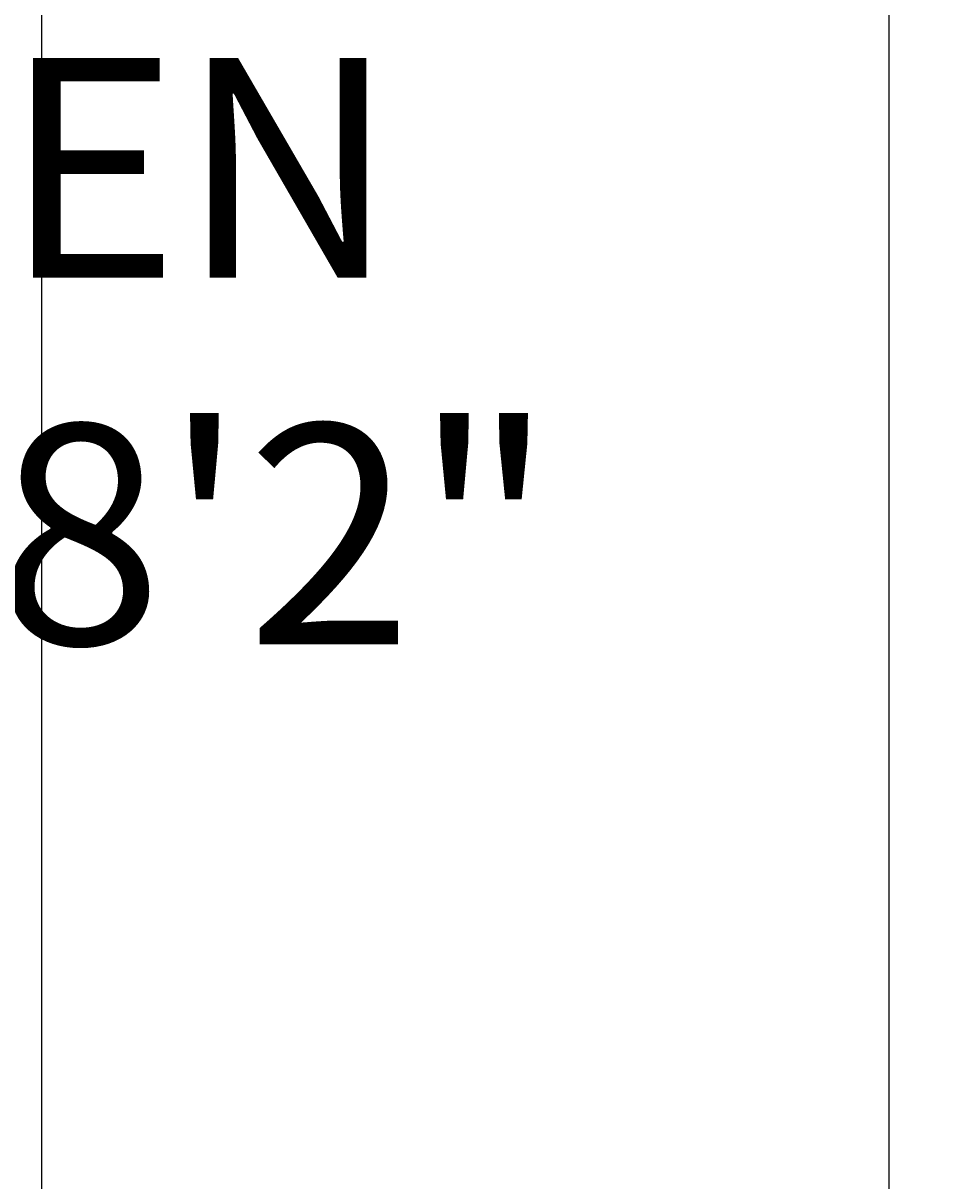
# Model space of a CAD drawing. Units: inches. Extents: x 37 to 824, y -700 to 234.
# Tile 32 of 77: x 227 to 251, y -237 to -206. Entities that reach past the tile are written whole.
import ezdxf

# ---------------------------------------------------------------- set-up
doc = ezdxf.new("R2010")
doc.units = ezdxf.units.IN
doc.header["$MEASUREMENT"] = 0
doc.layers.add('A-ANNO-DIMS', color=2, linetype='Continuous', lineweight=18)
doc.layers.add('A-AREA-IDEN', color=3, linetype='Continuous', lineweight=18)
doc.styles.get("Standard").update_dxf_attribs({"font": 'arial.ttf'})
doc.dimstyles.get("Standard").update_dxf_attribs({"dimtxt": 0.18, "dimasz": 0.18, "dimexe": 0.18, "dimexo": 0.0625, "dimgap": 0.09, "dimtad": 0, "dimtih": 1, "dimtoh": 1, "dimdec": 1, "dimzin": 0, "dimdsep": 46, "dimlunit": 4, "dimtxsty": 'Standard', "dimcen": 0.09, "dimadec": 0, "dimazin": 0, "dimtfac": 1, "dimtdec": 1, "dimtofl": 0, "dimtmove": 0, "dimatfit": 3, "dimfxl": 1, "dimtolj": 1, "dimtzin": 0, "dimarcsym": 0})

# ---------------------------------------------------------------- blocks, each defined once
blk = doc.blocks.new('*D77')
at = {"layer": 'A-ANNO-DIMS', "color": 0, "lineweight": -2, "ltscale": 0.5, "transparency": 16777216}
for p, q in [((227.077, 45.5), (227.077, -400.406)), ((290.077, 15.028), (290.077, -400.406)), ((227.257, -400.226), (258.248, -400.226)), ((289.897, -400.226), (258.906, -400.226))]:
    blk.add_line(p, q, dxfattribs=at)
at = {"layer": 'A-ANNO-DIMS', "color": 0, "ltscale": 0.5, "transparency": 16777216}
for points in [[(227.257, -400.196), (227.257, -400.256), (227.077, -400.226)], [(289.897, -400.196), (289.897, -400.256), (290.077, -400.226)]]:
    blk.add_solid(points, dxfattribs=at)
at = {"layer": 'Defpoints', "color": 0, "ltscale": 0.5, "transparency": 16777216}
for p in [(227.077, 45.563), (290.077, 15.09), (290.077, -400.226)]:
    blk.add_point(p, dxfattribs=at)
at = {"layer": 'A-ANNO-DIMS', "color": 0, "ltscale": 0.5, "transparency": 16777216, "insert": (258.577, -400.226), "char_height": 0.18, "attachment_point": 5}
blk.add_mtext('\\A1;5\'-3"', dxfattribs=at)
blk = doc.blocks.new('*D80')
at = {"layer": 'A-ANNO-DIMS', "color": 0, "lineweight": -2, "ltscale": 0.5, "transparency": 16777216}
for p, q in [((170.077, -167.972), (170.077, -400.406)), ((250.19, -167.972), (250.19, -400.406)), ((170.257, -400.226), (209.804, -400.226)), ((250.01, -400.226), (210.463, -400.226))]:
    blk.add_line(p, q, dxfattribs=at)
at = {"layer": 'A-ANNO-DIMS', "color": 0, "ltscale": 0.5, "transparency": 16777216}
for points in [[(170.257, -400.196), (170.257, -400.256), (170.077, -400.226)], [(250.01, -400.196), (250.01, -400.256), (250.19, -400.226)]]:
    blk.add_solid(points, dxfattribs=at)
at = {"layer": 'Defpoints', "color": 0, "ltscale": 0.5, "transparency": 16777216}
for p in [(170.077, -167.91), (250.19, -167.91), (250.19, -400.226)]:
    blk.add_point(p, dxfattribs=at)
at = {"layer": 'A-ANNO-DIMS', "color": 0, "ltscale": 0.5, "transparency": 16777216, "insert": (210.133, -400.226), "char_height": 0.18, "attachment_point": 5}
blk.add_mtext('\\A1;6\'-8"', dxfattribs=at)
blk = doc.blocks.new('*D81')
at = {"layer": 'A-ANNO-DIMS', "color": 0, "lineweight": -2, "ltscale": 0.5, "transparency": 16777216}
for p, q in [((290.077, -164.972), (290.077, -400.406)), ((250.19, -167.972), (250.19, -400.406)), ((250.37, -400.226), (269.804, -400.226)), ((289.897, -400.226), (270.463, -400.226))]:
    blk.add_line(p, q, dxfattribs=at)
at = {"layer": 'A-ANNO-DIMS', "color": 0, "ltscale": 0.5, "transparency": 16777216}
for points in [[(250.37, -400.196), (250.37, -400.256), (250.19, -400.226)], [(289.897, -400.196), (289.897, -400.256), (290.077, -400.226)]]:
    blk.add_solid(points, dxfattribs=at)
at = {"layer": 'Defpoints', "color": 0, "ltscale": 0.5, "transparency": 16777216}
for p in [(290.077, -164.91), (250.19, -167.91), (290.077, -400.226)]:
    blk.add_point(p, dxfattribs=at)
at = {"layer": 'A-ANNO-DIMS', "color": 0, "ltscale": 0.5, "transparency": 16777216, "insert": (270.133, -400.226), "char_height": 0.18, "attachment_point": 5}
blk.add_mtext('\\A1;3\'-4"', dxfattribs=at)
blk = doc.blocks.new('*D87')
at = {"layer": 'A-ANNO-DIMS', "color": 0, "lineweight": -2, "ltscale": 0.5, "transparency": 16777216}
for p, q in [((216.077, -356.847), (216.077, 234.17)), ((296.077, -356.847), (296.077, 234.17)), ((216.257, 233.99), (255.747, 233.99)), ((295.897, 233.99), (256.407, 233.99))]:
    blk.add_line(p, q, dxfattribs=at)
at = {"layer": 'A-ANNO-DIMS', "color": 0, "ltscale": 0.5, "transparency": 16777216}
for points in [[(216.257, 234.02), (216.257, 233.96), (216.077, 233.99)], [(295.897, 234.02), (295.897, 233.96), (296.077, 233.99)]]:
    blk.add_solid(points, dxfattribs=at)
at = {"layer": 'Defpoints', "color": 0, "ltscale": 0.5, "transparency": 16777216}
for p in [(296.077, 233.99), (216.077, -356.91), (296.077, -356.91)]:
    blk.add_point(p, dxfattribs=at)
at = {"layer": 'A-ANNO-DIMS', "color": 0, "ltscale": 0.5, "transparency": 16777216, "insert": (256.077, 233.99), "char_height": 0.18, "attachment_point": 5}
blk.add_mtext('\\A1;6\'-8"', dxfattribs=at)

msp = doc.modelspace()

# ---------------------------------------------------------------- texts
at = {"layer": 'A-AREA-IDEN', "insert": (202.252, -206.696), "char_height": 6, "attachment_point": 1}
msp.add_mtext_dynamic_manual_height_columns('KITCHEN\\P7\'6" X 8\'2"', width=88.32168, gutter_width=1, heights=[0], dxfattribs=at)

# ---------------------------------------------------------------- dimensions: what is measured, and where the dimension line sits
at = {"layer": 'A-ANNO-DIMS', "ltscale": 0.5}
for base, p1, p2, picture, middle in [((296.077, 233.99), (216.077, -356.91), (296.077, -356.91), '*D87', (256.077, 233.99)), ((290.077, -400.226), (227.077, 45.563), (290.077, 15.09), '*D77', (258.577, -400.226)), ((290.077, -400.226), (250.19, -167.91), (290.077, -164.91), '*D81', (270.133, -400.226)), ((250.19, -400.226), (170.077, -167.91), (250.19, -167.91), '*D80', (210.133, -400.226))]:
    dim = msp.add_linear_dim(base=base, p1=p1, p2=p2, dimstyle='Standard', override={"dimdec": 1, "dimlfac": 1, "dimrnd": 0, "dimzin": 1, "dimdsep": 46, "dimlunit": 4, "dimfrac": 2}, dxfattribs=at)
    dim.commit()
    dim.dimension.update_dxf_attribs({"geometry": picture, "text_midpoint": middle})

doc.saveas('drawing.dxf')
